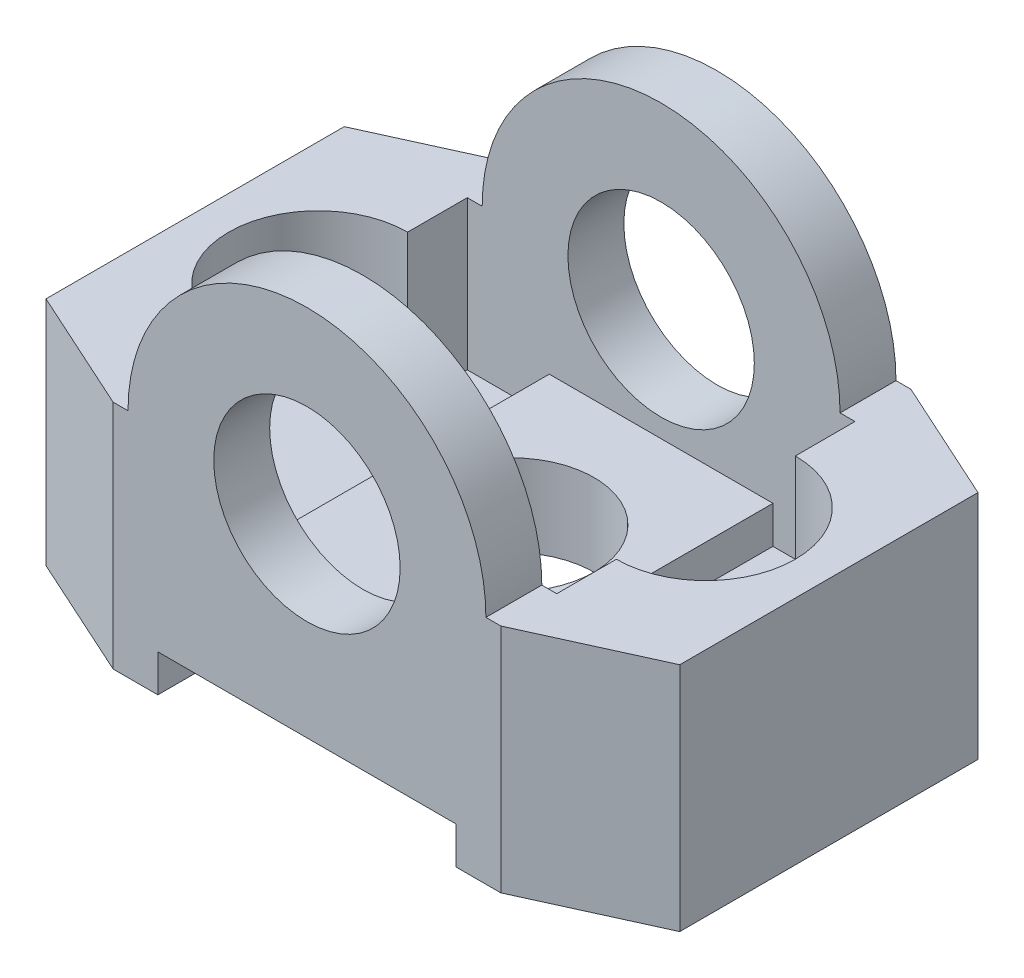
ISO-10303-21;
HEADER;
FILE_DESCRIPTION(('STEP AP214'),'2;1');
FILE_NAME('part.step','',(''),(''),'','','');
FILE_SCHEMA(('AUTOMOTIVE_DESIGN { 1 0 10303 214 1 1 1 1 }'));
ENDSEC;
DATA;
#1=APPLICATION_CONTEXT('core data for automotive mechanical design processes');
#2=APPLICATION_PROTOCOL_DEFINITION('international standard','automotive_design',2000,#1);
#3=PRODUCT_CONTEXT('',#1,'mechanical');
#4=PRODUCT('Part','Part','',(#3));
#5=PRODUCT_RELATED_PRODUCT_CATEGORY('part','',(#4));
#6=PRODUCT_DEFINITION_FORMATION('','',#4);
#7=PRODUCT_DEFINITION_CONTEXT('part definition',#1,'design');
#8=PRODUCT_DEFINITION('design','',#6,#7);
#9=PRODUCT_DEFINITION_SHAPE('','',#8);
#10=(LENGTH_UNIT() NAMED_UNIT(*) SI_UNIT(.MILLI.,.METRE.));
#11=(NAMED_UNIT(*) PLANE_ANGLE_UNIT() SI_UNIT($,.RADIAN.));
#12=(NAMED_UNIT(*) SI_UNIT($,.STERADIAN.) SOLID_ANGLE_UNIT());
#13=UNCERTAINTY_MEASURE_WITH_UNIT(LENGTH_MEASURE(1.E-05),#10,'distance_accuracy_value','');
#14=(GEOMETRIC_REPRESENTATION_CONTEXT(3) GLOBAL_UNCERTAINTY_ASSIGNED_CONTEXT((#13)) GLOBAL_UNIT_ASSIGNED_CONTEXT((#10,
#11,#12)) REPRESENTATION_CONTEXT('',''));
#15=CARTESIAN_POINT('',(0.,0.,0.));
#16=DIRECTION('',(0.,0.,1.));
#17=DIRECTION('',(1.,0.,0.));
#18=AXIS2_PLACEMENT_3D('',#15,#16,#17);
#19=CARTESIAN_POINT('',(0.,0.,0.));
#20=DIRECTION('',(0.,-1.,0.));
#21=DIRECTION('',(0.,0.,-1.));
#22=AXIS2_PLACEMENT_3D('',#19,#20,#21);
#23=PLANE('',#22);
#24=DIRECTION('',(0.,0.,1.));
#25=VECTOR('',#24,1.);
#26=CARTESIAN_POINT('',(-20.,0.,-27.501));
#27=LINE('',#26,#25);
#28=CARTESIAN_POINT('',(-20.,0.,-27.5));
#29=VERTEX_POINT('',#28);
#30=CARTESIAN_POINT('',(-20.,0.,27.5));
#31=VERTEX_POINT('',#30);
#32=EDGE_CURVE('E223',#29,#31,#27,.T.);
#33=ORIENTED_EDGE('',*,*,#32,.T.);
#34=DIRECTION('',(1.,0.,0.));
#35=VECTOR('',#34,1.);
#36=CARTESIAN_POINT('',(26.,0.,27.5));
#37=LINE('',#36,#35);
#38=CARTESIAN_POINT('',(-26.,0.,27.5));
#39=VERTEX_POINT('',#38);
#40=EDGE_CURVE('E267',#39,#31,#37,.T.);
#41=ORIENTED_EDGE('',*,*,#40,.F.);
#42=DIRECTION('',(0.910366477462604,0.,0.413802944301187));
#43=VECTOR('',#42,1.);
#44=CARTESIAN_POINT('',(-42.5,0.,20.));
#45=LINE('',#44,#43);
#46=CARTESIAN_POINT('',(-42.5,0.,20.));
#47=VERTEX_POINT('',#46);
#48=EDGE_CURVE('E264',#47,#39,#45,.T.);
#49=ORIENTED_EDGE('',*,*,#48,.F.);
#50=DIRECTION('',(0.,0.,1.));
#51=VECTOR('',#50,1.);
#52=CARTESIAN_POINT('',(-42.5,0.,-20.));
#53=LINE('',#52,#51);
#54=CARTESIAN_POINT('',(-42.5,0.,-20.));
#55=VERTEX_POINT('',#54);
#56=EDGE_CURVE('E265',#55,#47,#53,.T.);
#57=ORIENTED_EDGE('',*,*,#56,.F.);
#58=DIRECTION('',(-0.910366477462604,0.,0.413802944301186));
#59=VECTOR('',#58,1.);
#60=CARTESIAN_POINT('',(-26.,0.,-27.5));
#61=LINE('',#60,#59);
#62=CARTESIAN_POINT('',(-26.,0.,-27.5));
#63=VERTEX_POINT('',#62);
#64=EDGE_CURVE('E253',#63,#55,#61,.T.);
#65=ORIENTED_EDGE('',*,*,#64,.F.);
#66=DIRECTION('',(-1.,0.,0.));
#67=VECTOR('',#66,1.);
#68=CARTESIAN_POINT('',(-26.,0.,-27.5));
#69=LINE('',#68,#67);
#70=EDGE_CURVE('E244',#29,#63,#69,.T.);
#71=ORIENTED_EDGE('',*,*,#70,.F.);
#72=EDGE_LOOP('',(#33,#41,#49,#57,#65,#71));
#73=FACE_BOUND('',#72,.T.);
#74=ADVANCED_FACE('F39',(#73),#23,.T.);
#75=CARTESIAN_POINT('',(-26.,31.,-20.));
#76=DIRECTION('',(0.,0.,1.));
#77=DIRECTION('',(1.,0.,0.));
#78=AXIS2_PLACEMENT_3D('',#75,#76,#77);
#79=PLANE('',#78);
#80=CARTESIAN_POINT('',(0.,31.,-20.));
#81=DIRECTION('',(0.,0.,1.));
#82=DIRECTION('',(1.,0.,0.));
#83=AXIS2_PLACEMENT_3D('',#80,#81,#82);
#84=CIRCLE('',#83,12.5);
#85=CARTESIAN_POINT('',(12.5,31.,-20.));
#86=VERTEX_POINT('',#85);
#87=EDGE_CURVE('E297',#86,#86,#84,.T.);
#88=ORIENTED_EDGE('',*,*,#87,.F.);
#89=EDGE_LOOP('',(#88));
#90=FACE_BOUND('',#89,.T.);
#91=DIRECTION('',(-1.,0.,0.));
#92=VECTOR('',#91,1.);
#93=CARTESIAN_POINT('',(-15.,16.,-20.));
#94=LINE('',#93,#92);
#95=CARTESIAN_POINT('',(15.,16.,-20.));
#96=VERTEX_POINT('',#95);
#97=CARTESIAN_POINT('',(-15.,16.,-20.));
#98=VERTEX_POINT('',#97);
#99=EDGE_CURVE('E422',#96,#98,#94,.T.);
#100=ORIENTED_EDGE('',*,*,#99,.F.);
#101=DIRECTION('',(0.,-1.,0.));
#102=VECTOR('',#101,1.);
#103=CARTESIAN_POINT('',(15.,16.,-20.));
#104=LINE('',#103,#102);
#105=CARTESIAN_POINT('',(15.,11.,-20.));
#106=VERTEX_POINT('',#105);
#107=EDGE_CURVE('E439',#96,#106,#104,.T.);
#108=ORIENTED_EDGE('',*,*,#107,.T.);
#109=DIRECTION('',(-1.,0.,0.));
#110=VECTOR('',#109,1.);
#111=CARTESIAN_POINT('',(-26.,11.,-20.));
#112=LINE('',#111,#110);
#113=CARTESIAN_POINT('',(26.,11.,-20.));
#114=VERTEX_POINT('',#113);
#115=EDGE_CURVE('E459',#114,#106,#112,.T.);
#116=ORIENTED_EDGE('',*,*,#115,.F.);
#117=DIRECTION('',(0.,-1.,0.));
#118=VECTOR('',#117,1.);
#119=CARTESIAN_POINT('',(26.,31.,-20.));
#120=LINE('',#119,#118);
#121=CARTESIAN_POINT('',(26.,31.,-20.));
#122=VERTEX_POINT('',#121);
#123=EDGE_CURVE('E260',#122,#114,#120,.T.);
#124=ORIENTED_EDGE('',*,*,#123,.F.);
#125=DIRECTION('',(-1.,0.,0.));
#126=VECTOR('',#125,1.);
#127=CARTESIAN_POINT('',(-26.,31.,-20.));
#128=LINE('',#127,#126);
#129=CARTESIAN_POINT('',(24.,31.,-20.));
#130=VERTEX_POINT('',#129);
#131=EDGE_CURVE('E337',#122,#130,#128,.T.);
#132=ORIENTED_EDGE('',*,*,#131,.T.);
#133=CARTESIAN_POINT('',(0.,31.,-20.));
#134=DIRECTION('',(0.,0.,1.));
#135=DIRECTION('',(1.,0.,0.));
#136=AXIS2_PLACEMENT_3D('',#133,#134,#135);
#137=CIRCLE('',#136,24.);
#138=CARTESIAN_POINT('',(-24.,31.,-20.));
#139=VERTEX_POINT('',#138);
#140=EDGE_CURVE('E320',#139,#130,#137,.F.);
#141=ORIENTED_EDGE('',*,*,#140,.F.);
#142=CARTESIAN_POINT('',(-26.,31.,-20.));
#143=VERTEX_POINT('',#142);
#144=EDGE_CURVE('E333',#139,#143,#128,.T.);
#145=ORIENTED_EDGE('',*,*,#144,.T.);
#146=DIRECTION('',(0.,-1.,0.));
#147=VECTOR('',#146,1.);
#148=CARTESIAN_POINT('',(-26.,31.,-20.));
#149=LINE('',#148,#147);
#150=CARTESIAN_POINT('',(-26.,11.,-20.));
#151=VERTEX_POINT('',#150);
#152=EDGE_CURVE('E371',#143,#151,#149,.T.);
#153=ORIENTED_EDGE('',*,*,#152,.T.);
#154=CARTESIAN_POINT('',(-15.,11.,-20.));
#155=VERTEX_POINT('',#154);
#156=EDGE_CURVE('E456',#155,#151,#112,.T.);
#157=ORIENTED_EDGE('',*,*,#156,.F.);
#158=DIRECTION('',(0.,-1.,0.));
#159=VECTOR('',#158,1.);
#160=CARTESIAN_POINT('',(-15.,16.,-20.));
#161=LINE('',#160,#159);
#162=EDGE_CURVE('E64',#98,#155,#161,.T.);
#163=ORIENTED_EDGE('',*,*,#162,.F.);
#164=EDGE_LOOP('',(#100,#108,#116,#124,#132,#141,#145,#153,#157,#163));
#165=FACE_BOUND('',#164,.T.);
#166=ADVANCED_FACE('F474',(#90,#165),#79,.T.);
#167=CARTESIAN_POINT('',(26.,31.,20.));
#168=DIRECTION('',(0.,0.,-1.));
#169=DIRECTION('',(-1.,0.,0.));
#170=AXIS2_PLACEMENT_3D('',#167,#168,#169);
#171=PLANE('',#170);
#172=CARTESIAN_POINT('',(0.,31.,20.));
#173=DIRECTION('',(0.,0.,-1.));
#174=DIRECTION('',(-1.,0.,0.));
#175=AXIS2_PLACEMENT_3D('',#172,#173,#174);
#176=CIRCLE('',#175,12.5);
#177=CARTESIAN_POINT('',(-12.5,31.,20.));
#178=VERTEX_POINT('',#177);
#179=EDGE_CURVE('E294',#178,#178,#176,.T.);
#180=ORIENTED_EDGE('',*,*,#179,.F.);
#181=EDGE_LOOP('',(#180));
#182=FACE_BOUND('',#181,.T.);
#183=DIRECTION('',(1.,0.,0.));
#184=VECTOR('',#183,1.);
#185=CARTESIAN_POINT('',(26.,11.,20.));
#186=LINE('',#185,#184);
#187=CARTESIAN_POINT('',(15.,11.,20.));
#188=VERTEX_POINT('',#187);
#189=CARTESIAN_POINT('',(26.,11.,20.));
#190=VERTEX_POINT('',#189);
#191=EDGE_CURVE('E447',#188,#190,#186,.T.);
#192=ORIENTED_EDGE('',*,*,#191,.F.);
#193=DIRECTION('',(0.,-1.,0.));
#194=VECTOR('',#193,1.);
#195=CARTESIAN_POINT('',(15.,16.,20.));
#196=LINE('',#195,#194);
#197=CARTESIAN_POINT('',(15.,16.,20.));
#198=VERTEX_POINT('',#197);
#199=EDGE_CURVE('E435',#198,#188,#196,.T.);
#200=ORIENTED_EDGE('',*,*,#199,.F.);
#201=DIRECTION('',(1.,0.,0.));
#202=VECTOR('',#201,1.);
#203=CARTESIAN_POINT('',(-15.,16.,20.));
#204=LINE('',#203,#202);
#205=CARTESIAN_POINT('',(-15.,16.,20.));
#206=VERTEX_POINT('',#205);
#207=EDGE_CURVE('E429',#206,#198,#204,.T.);
#208=ORIENTED_EDGE('',*,*,#207,.F.);
#209=DIRECTION('',(0.,-1.,0.));
#210=VECTOR('',#209,1.);
#211=CARTESIAN_POINT('',(-15.,16.,20.));
#212=LINE('',#211,#210);
#213=CARTESIAN_POINT('',(-15.,11.,20.));
#214=VERTEX_POINT('',#213);
#215=EDGE_CURVE('E436',#206,#214,#212,.T.);
#216=ORIENTED_EDGE('',*,*,#215,.T.);
#217=CARTESIAN_POINT('',(-26.,11.,20.));
#218=VERTEX_POINT('',#217);
#219=EDGE_CURVE('E449',#218,#214,#186,.T.);
#220=ORIENTED_EDGE('',*,*,#219,.F.);
#221=DIRECTION('',(0.,-1.,0.));
#222=VECTOR('',#221,1.);
#223=CARTESIAN_POINT('',(-26.,31.,20.));
#224=LINE('',#223,#222);
#225=CARTESIAN_POINT('',(-26.,31.,20.));
#226=VERTEX_POINT('',#225);
#227=EDGE_CURVE('E362',#226,#218,#224,.T.);
#228=ORIENTED_EDGE('',*,*,#227,.F.);
#229=DIRECTION('',(1.,0.,0.));
#230=VECTOR('',#229,1.);
#231=CARTESIAN_POINT('',(26.,31.,20.));
#232=LINE('',#231,#230);
#233=CARTESIAN_POINT('',(-24.,31.,20.));
#234=VERTEX_POINT('',#233);
#235=EDGE_CURVE('E347',#226,#234,#232,.T.);
#236=ORIENTED_EDGE('',*,*,#235,.T.);
#237=CARTESIAN_POINT('',(0.,31.,20.));
#238=DIRECTION('',(0.,0.,-1.));
#239=DIRECTION('',(-1.,0.,0.));
#240=AXIS2_PLACEMENT_3D('',#237,#238,#239);
#241=CIRCLE('',#240,24.);
#242=CARTESIAN_POINT('',(24.,31.,20.));
#243=VERTEX_POINT('',#242);
#244=EDGE_CURVE('E330',#243,#234,#241,.F.);
#245=ORIENTED_EDGE('',*,*,#244,.F.);
#246=CARTESIAN_POINT('',(26.,31.,20.));
#247=VERTEX_POINT('',#246);
#248=EDGE_CURVE('E341',#243,#247,#232,.T.);
#249=ORIENTED_EDGE('',*,*,#248,.T.);
#250=DIRECTION('',(0.,-1.,0.));
#251=VECTOR('',#250,1.);
#252=CARTESIAN_POINT('',(26.,31.,20.));
#253=LINE('',#252,#251);
#254=EDGE_CURVE('E359',#247,#190,#253,.T.);
#255=ORIENTED_EDGE('',*,*,#254,.T.);
#256=EDGE_LOOP('',(#192,#200,#208,#216,#220,#228,#236,#245,#249,#255));
#257=FACE_BOUND('',#256,.T.);
#258=ADVANCED_FACE('F495',(#182,#257),#171,.T.);
#259=CARTESIAN_POINT('',(0.,11.,0.));
#260=DIRECTION('',(0.,1.,0.));
#261=DIRECTION('',(0.,0.,1.));
#262=AXIS2_PLACEMENT_3D('',#259,#260,#261);
#263=PLANE('',#262);
#264=ORIENTED_EDGE('',*,*,#115,.T.);
#265=DIRECTION('',(0.,0.,-1.));
#266=VECTOR('',#265,1.);
#267=CARTESIAN_POINT('',(15.,11.,20.));
#268=LINE('',#267,#266);
#269=EDGE_CURVE('E423',#188,#106,#268,.T.);
#270=ORIENTED_EDGE('',*,*,#269,.F.);
#271=ORIENTED_EDGE('',*,*,#191,.T.);
#272=DIRECTION('',(0.,0.,-1.));
#273=VECTOR('',#272,1.);
#274=CARTESIAN_POINT('',(26.,11.,12.));
#275=LINE('',#274,#273);
#276=CARTESIAN_POINT('',(26.,11.,12.));
#277=VERTEX_POINT('',#276);
#278=EDGE_CURVE('E444',#190,#277,#275,.T.);
#279=ORIENTED_EDGE('',*,*,#278,.T.);
#280=CARTESIAN_POINT('',(26.,11.,0.));
#281=DIRECTION('',(0.,1.,0.));
#282=DIRECTION('',(0.,0.,1.));
#283=AXIS2_PLACEMENT_3D('',#280,#281,#282);
#284=CIRCLE('',#283,12.);
#285=CARTESIAN_POINT('',(26.,11.,-12.));
#286=VERTEX_POINT('',#285);
#287=EDGE_CURVE('E11',#277,#286,#284,.T.);
#288=ORIENTED_EDGE('',*,*,#287,.T.);
#289=DIRECTION('',(0.,0.,-1.));
#290=VECTOR('',#289,1.);
#291=CARTESIAN_POINT('',(26.,11.,-20.));
#292=LINE('',#291,#290);
#293=EDGE_CURVE('E310',#286,#114,#292,.T.);
#294=ORIENTED_EDGE('',*,*,#293,.T.);
#295=EDGE_LOOP('',(#264,#270,#271,#279,#288,#294));
#296=FACE_BOUND('',#295,.T.);
#297=ADVANCED_FACE('F516',(#296),#263,.T.);
#298=ORIENTED_EDGE('',*,*,#219,.T.);
#299=DIRECTION('',(0.,0.,1.));
#300=VECTOR('',#299,1.);
#301=CARTESIAN_POINT('',(-15.,11.,20.));
#302=LINE('',#301,#300);
#303=EDGE_CURVE('E426',#155,#214,#302,.T.);
#304=ORIENTED_EDGE('',*,*,#303,.F.);
#305=ORIENTED_EDGE('',*,*,#156,.T.);
#306=DIRECTION('',(0.,0.,1.));
#307=VECTOR('',#306,1.);
#308=CARTESIAN_POINT('',(-26.,11.,-12.));
#309=LINE('',#308,#307);
#310=CARTESIAN_POINT('',(-26.,11.,-12.));
#311=VERTEX_POINT('',#310);
#312=EDGE_CURVE('E457',#151,#311,#309,.T.);
#313=ORIENTED_EDGE('',*,*,#312,.T.);
#314=CARTESIAN_POINT('',(-26.,11.,0.));
#315=DIRECTION('',(0.,1.,0.));
#316=DIRECTION('',(0.,0.,1.));
#317=AXIS2_PLACEMENT_3D('',#314,#315,#316);
#318=CIRCLE('',#317,12.);
#319=CARTESIAN_POINT('',(-26.,11.,12.));
#320=VERTEX_POINT('',#319);
#321=EDGE_CURVE('E453',#311,#320,#318,.T.);
#322=ORIENTED_EDGE('',*,*,#321,.T.);
#323=DIRECTION('',(0.,0.,1.));
#324=VECTOR('',#323,1.);
#325=CARTESIAN_POINT('',(-26.,11.,20.));
#326=LINE('',#325,#324);
#327=EDGE_CURVE('E448',#320,#218,#326,.T.);
#328=ORIENTED_EDGE('',*,*,#327,.T.);
#329=EDGE_LOOP('',(#298,#304,#305,#313,#322,#328));
#330=FACE_BOUND('',#329,.T.);
#331=ADVANCED_FACE('F470',(#330),#263,.T.);
#332=CARTESIAN_POINT('',(0.,31.,0.));
#333=DIRECTION('',(0.,-1.,0.));
#334=DIRECTION('',(0.,0.,-1.));
#335=AXIS2_PLACEMENT_3D('',#332,#333,#334);
#336=PLANE('',#335);
#337=ORIENTED_EDGE('',*,*,#144,.F.);
#338=DIRECTION('',(0.,0.,-1.));
#339=VECTOR('',#338,1.);
#340=CARTESIAN_POINT('',(-24.,31.,33.665631459995));
#341=LINE('',#340,#339);
#342=CARTESIAN_POINT('',(-24.,31.,-27.5));
#343=VERTEX_POINT('',#342);
#344=EDGE_CURVE('E316',#139,#343,#341,.T.);
#345=ORIENTED_EDGE('',*,*,#344,.T.);
#346=DIRECTION('',(-1.,0.,0.));
#347=VECTOR('',#346,1.);
#348=CARTESIAN_POINT('',(-26.,31.,-27.5));
#349=LINE('',#348,#347);
#350=CARTESIAN_POINT('',(-26.,31.,-27.5));
#351=VERTEX_POINT('',#350);
#352=EDGE_CURVE('E378',#343,#351,#349,.T.);
#353=ORIENTED_EDGE('',*,*,#352,.T.);
#354=DIRECTION('',(-0.910366477462604,0.,0.413802944301186));
#355=VECTOR('',#354,1.);
#356=CARTESIAN_POINT('',(-26.,31.,-27.5));
#357=LINE('',#356,#355);
#358=CARTESIAN_POINT('',(-42.5,31.,-20.));
#359=VERTEX_POINT('',#358);
#360=EDGE_CURVE('E385',#351,#359,#357,.T.);
#361=ORIENTED_EDGE('',*,*,#360,.T.);
#362=DIRECTION('',(0.,0.,1.));
#363=VECTOR('',#362,1.);
#364=CARTESIAN_POINT('',(-42.5,31.,-20.));
#365=LINE('',#364,#363);
#366=CARTESIAN_POINT('',(-42.5,31.,20.));
#367=VERTEX_POINT('',#366);
#368=EDGE_CURVE('E383',#359,#367,#365,.T.);
#369=ORIENTED_EDGE('',*,*,#368,.T.);
#370=DIRECTION('',(0.910366477462604,0.,0.413802944301187));
#371=VECTOR('',#370,1.);
#372=CARTESIAN_POINT('',(-42.5,31.,20.));
#373=LINE('',#372,#371);
#374=CARTESIAN_POINT('',(-26.,31.,27.5));
#375=VERTEX_POINT('',#374);
#376=EDGE_CURVE('E387',#367,#375,#373,.T.);
#377=ORIENTED_EDGE('',*,*,#376,.T.);
#378=DIRECTION('',(1.,0.,0.));
#379=VECTOR('',#378,1.);
#380=CARTESIAN_POINT('',(26.,31.,27.5));
#381=LINE('',#380,#379);
#382=CARTESIAN_POINT('',(-24.,31.,27.5));
#383=VERTEX_POINT('',#382);
#384=EDGE_CURVE('E386',#375,#383,#381,.T.);
#385=ORIENTED_EDGE('',*,*,#384,.T.);
#386=DIRECTION('',(0.,0.,1.));
#387=VECTOR('',#386,1.);
#388=CARTESIAN_POINT('',(-24.,31.,-33.6656314599949));
#389=LINE('',#388,#387);
#390=EDGE_CURVE('E328',#234,#383,#389,.T.);
#391=ORIENTED_EDGE('',*,*,#390,.F.);
#392=ORIENTED_EDGE('',*,*,#235,.F.);
#393=DIRECTION('',(0.,0.,1.));
#394=VECTOR('',#393,1.);
#395=CARTESIAN_POINT('',(-26.,31.,20.));
#396=LINE('',#395,#394);
#397=CARTESIAN_POINT('',(-26.,31.,12.));
#398=VERTEX_POINT('',#397);
#399=EDGE_CURVE('E343',#398,#226,#396,.T.);
#400=ORIENTED_EDGE('',*,*,#399,.F.);
#401=CARTESIAN_POINT('',(-26.,31.,0.));
#402=DIRECTION('',(0.,1.,0.));
#403=DIRECTION('',(0.,0.,1.));
#404=AXIS2_PLACEMENT_3D('',#401,#402,#403);
#405=CIRCLE('',#404,12.);
#406=CARTESIAN_POINT('',(-26.,31.,-12.));
#407=VERTEX_POINT('',#406);
#408=EDGE_CURVE('E342',#407,#398,#405,.T.);
#409=ORIENTED_EDGE('',*,*,#408,.F.);
#410=DIRECTION('',(0.,0.,1.));
#411=VECTOR('',#410,1.);
#412=CARTESIAN_POINT('',(-26.,31.,-12.));
#413=LINE('',#412,#411);
#414=EDGE_CURVE('E336',#143,#407,#413,.T.);
#415=ORIENTED_EDGE('',*,*,#414,.F.);
#416=EDGE_LOOP('',(#337,#345,#353,#361,#369,#377,#385,#391,#392,#400,#409,#415));
#417=FACE_BOUND('',#416,.T.);
#418=ADVANCED_FACE('F479',(#417),#336,.F.);
#419=CARTESIAN_POINT('',(26.,31.,-27.5));
#420=VERTEX_POINT('',#419);
#421=CARTESIAN_POINT('',(24.,31.,-27.5));
#422=VERTEX_POINT('',#421);
#423=EDGE_CURVE('E377',#420,#422,#349,.T.);
#424=ORIENTED_EDGE('',*,*,#423,.T.);
#425=DIRECTION('',(0.,0.,-1.));
#426=VECTOR('',#425,1.);
#427=CARTESIAN_POINT('',(24.,31.,33.665631459995));
#428=LINE('',#427,#426);
#429=EDGE_CURVE('E317',#130,#422,#428,.T.);
#430=ORIENTED_EDGE('',*,*,#429,.F.);
#431=ORIENTED_EDGE('',*,*,#131,.F.);
#432=DIRECTION('',(0.,0.,-1.));
#433=VECTOR('',#432,1.);
#434=CARTESIAN_POINT('',(26.,31.,-20.));
#435=LINE('',#434,#433);
#436=CARTESIAN_POINT('',(26.,31.,-12.));
#437=VERTEX_POINT('',#436);
#438=EDGE_CURVE('E334',#437,#122,#435,.T.);
#439=ORIENTED_EDGE('',*,*,#438,.F.);
#440=CARTESIAN_POINT('',(26.,31.,0.));
#441=DIRECTION('',(0.,1.,0.));
#442=DIRECTION('',(0.,0.,-1.));
#443=AXIS2_PLACEMENT_3D('',#440,#441,#442);
#444=CIRCLE('',#443,12.);
#445=CARTESIAN_POINT('',(26.,31.,12.));
#446=VERTEX_POINT('',#445);
#447=EDGE_CURVE('E354',#446,#437,#444,.T.);
#448=ORIENTED_EDGE('',*,*,#447,.F.);
#449=DIRECTION('',(0.,0.,-1.));
#450=VECTOR('',#449,1.);
#451=CARTESIAN_POINT('',(26.,31.,12.));
#452=LINE('',#451,#450);
#453=EDGE_CURVE('E349',#247,#446,#452,.T.);
#454=ORIENTED_EDGE('',*,*,#453,.F.);
#455=ORIENTED_EDGE('',*,*,#248,.F.);
#456=DIRECTION('',(0.,0.,1.));
#457=VECTOR('',#456,1.);
#458=CARTESIAN_POINT('',(24.,31.,-33.6656314599949));
#459=LINE('',#458,#457);
#460=CARTESIAN_POINT('',(24.,31.,27.5));
#461=VERTEX_POINT('',#460);
#462=EDGE_CURVE('E326',#243,#461,#459,.T.);
#463=ORIENTED_EDGE('',*,*,#462,.T.);
#464=CARTESIAN_POINT('',(26.,31.,27.5));
#465=VERTEX_POINT('',#464);
#466=EDGE_CURVE('E389',#461,#465,#381,.T.);
#467=ORIENTED_EDGE('',*,*,#466,.T.);
#468=DIRECTION('',(0.910366477462605,0.,-0.413802944301184));
#469=VECTOR('',#468,1.);
#470=CARTESIAN_POINT('',(42.5,31.,20.));
#471=LINE('',#470,#469);
#472=CARTESIAN_POINT('',(42.5,31.,20.));
#473=VERTEX_POINT('',#472);
#474=EDGE_CURVE('E394',#465,#473,#471,.T.);
#475=ORIENTED_EDGE('',*,*,#474,.T.);
#476=DIRECTION('',(0.,0.,-1.));
#477=VECTOR('',#476,1.);
#478=CARTESIAN_POINT('',(42.5,31.,-20.));
#479=LINE('',#478,#477);
#480=CARTESIAN_POINT('',(42.5,31.,-20.));
#481=VERTEX_POINT('',#480);
#482=EDGE_CURVE('E282',#473,#481,#479,.T.);
#483=ORIENTED_EDGE('',*,*,#482,.T.);
#484=DIRECTION('',(-0.910366477462604,0.,-0.413802944301186));
#485=VECTOR('',#484,1.);
#486=CARTESIAN_POINT('',(26.,31.,-27.5));
#487=LINE('',#486,#485);
#488=EDGE_CURVE('E280',#481,#420,#487,.T.);
#489=ORIENTED_EDGE('',*,*,#488,.T.);
#490=EDGE_LOOP('',(#424,#430,#431,#439,#448,#454,#455,#463,#467,#475,#483,#489));
#491=FACE_BOUND('',#490,.T.);
#492=ADVANCED_FACE('F397',(#491),#336,.F.);
#493=DIRECTION('',(0.,0.,1.));
#494=VECTOR('',#493,1.);
#495=CARTESIAN_POINT('',(20.,0.,-27.501));
#496=LINE('',#495,#494);
#497=CARTESIAN_POINT('',(20.,0.,-27.5));
#498=VERTEX_POINT('',#497);
#499=CARTESIAN_POINT('',(20.,0.,27.5));
#500=VERTEX_POINT('',#499);
#501=EDGE_CURVE('E237',#498,#500,#496,.T.);
#502=ORIENTED_EDGE('',*,*,#501,.F.);
#503=CARTESIAN_POINT('',(26.,0.,-27.5));
#504=VERTEX_POINT('',#503);
#505=EDGE_CURVE('E252',#504,#498,#69,.T.);
#506=ORIENTED_EDGE('',*,*,#505,.F.);
#507=DIRECTION('',(-0.910366477462604,0.,-0.413802944301186));
#508=VECTOR('',#507,1.);
#509=CARTESIAN_POINT('',(26.,0.,-27.5));
#510=LINE('',#509,#508);
#511=CARTESIAN_POINT('',(42.5,0.,-20.));
#512=VERTEX_POINT('',#511);
#513=EDGE_CURVE('E251',#512,#504,#510,.T.);
#514=ORIENTED_EDGE('',*,*,#513,.F.);
#515=DIRECTION('',(0.,0.,-1.));
#516=VECTOR('',#515,1.);
#517=CARTESIAN_POINT('',(42.5,0.,-20.));
#518=LINE('',#517,#516);
#519=CARTESIAN_POINT('',(42.5,0.,20.));
#520=VERTEX_POINT('',#519);
#521=EDGE_CURVE('E273',#520,#512,#518,.T.);
#522=ORIENTED_EDGE('',*,*,#521,.F.);
#523=DIRECTION('',(0.910366477462605,0.,-0.413802944301184));
#524=VECTOR('',#523,1.);
#525=CARTESIAN_POINT('',(42.5,0.,20.));
#526=LINE('',#525,#524);
#527=CARTESIAN_POINT('',(26.,0.,27.5));
#528=VERTEX_POINT('',#527);
#529=EDGE_CURVE('E271',#528,#520,#526,.T.);
#530=ORIENTED_EDGE('',*,*,#529,.F.);
#531=EDGE_CURVE('E268',#500,#528,#37,.T.);
#532=ORIENTED_EDGE('',*,*,#531,.F.);
#533=EDGE_LOOP('',(#502,#506,#514,#522,#530,#532));
#534=FACE_BOUND('',#533,.T.);
#535=ADVANCED_FACE('F406',(#534),#23,.T.);
#536=CARTESIAN_POINT('',(26.,31.,-27.5));
#537=DIRECTION('',(-0.413802944301186,0.,0.910366477462604));
#538=DIRECTION('',(0.910366477462604,0.,0.413802944301186));
#539=AXIS2_PLACEMENT_3D('',#536,#537,#538);
#540=PLANE('',#539);
#541=DIRECTION('',(0.,-1.,0.));
#542=VECTOR('',#541,1.);
#543=CARTESIAN_POINT('',(42.5,31.,-20.));
#544=LINE('',#543,#542);
#545=EDGE_CURVE('E279',#481,#512,#544,.T.);
#546=ORIENTED_EDGE('',*,*,#545,.T.);
#547=ORIENTED_EDGE('',*,*,#513,.T.);
#548=DIRECTION('',(0.,-1.,0.));
#549=VECTOR('',#548,1.);
#550=CARTESIAN_POINT('',(26.,31.,-27.5));
#551=LINE('',#550,#549);
#552=EDGE_CURVE('E50',#420,#504,#551,.T.);
#553=ORIENTED_EDGE('',*,*,#552,.F.);
#554=ORIENTED_EDGE('',*,*,#488,.F.);
#555=EDGE_LOOP('',(#546,#547,#553,#554));
#556=FACE_BOUND('',#555,.T.);
#557=ADVANCED_FACE('F41',(#556),#540,.F.);
#558=CARTESIAN_POINT('',(-26.,31.,-27.5));
#559=DIRECTION('',(0.,0.,1.));
#560=DIRECTION('',(1.,0.,0.));
#561=AXIS2_PLACEMENT_3D('',#558,#559,#560);
#562=PLANE('',#561);
#563=CARTESIAN_POINT('',(0.,31.,-27.5));
#564=DIRECTION('',(0.,0.,1.));
#565=DIRECTION('',(1.,0.,0.));
#566=AXIS2_PLACEMENT_3D('',#563,#564,#565);
#567=CIRCLE('',#566,12.5);
#568=CARTESIAN_POINT('',(12.5,31.,-27.5));
#569=VERTEX_POINT('',#568);
#570=EDGE_CURVE('E299',#569,#569,#567,.T.);
#571=ORIENTED_EDGE('',*,*,#570,.T.);
#572=EDGE_LOOP('',(#571));
#573=FACE_BOUND('',#572,.T.);
#574=DIRECTION('',(1.,0.,0.));
#575=VECTOR('',#574,1.);
#576=CARTESIAN_POINT('',(-20.,5.,-27.5));
#577=LINE('',#576,#575);
#578=CARTESIAN_POINT('',(-20.,5.,-27.5));
#579=VERTEX_POINT('',#578);
#580=CARTESIAN_POINT('',(20.,5.,-27.5));
#581=VERTEX_POINT('',#580);
#582=EDGE_CURVE('E247',#579,#581,#577,.T.);
#583=ORIENTED_EDGE('',*,*,#582,.F.);
#584=DIRECTION('',(0.,1.,0.));
#585=VECTOR('',#584,1.);
#586=CARTESIAN_POINT('',(-20.,0.,-27.5));
#587=LINE('',#586,#585);
#588=EDGE_CURVE('E230',#29,#579,#587,.T.);
#589=ORIENTED_EDGE('',*,*,#588,.F.);
#590=ORIENTED_EDGE('',*,*,#70,.T.);
#591=DIRECTION('',(0.,-1.,0.));
#592=VECTOR('',#591,1.);
#593=CARTESIAN_POINT('',(-26.,31.,-27.5));
#594=LINE('',#593,#592);
#595=EDGE_CURVE('E295',#351,#63,#594,.T.);
#596=ORIENTED_EDGE('',*,*,#595,.F.);
#597=ORIENTED_EDGE('',*,*,#352,.F.);
#598=CARTESIAN_POINT('',(0.,31.,-27.5));
#599=DIRECTION('',(0.,0.,-1.));
#600=DIRECTION('',(1.,0.,0.));
#601=AXIS2_PLACEMENT_3D('',#598,#599,#600);
#602=CIRCLE('',#601,24.);
#603=EDGE_CURVE('E302',#343,#422,#602,.T.);
#604=ORIENTED_EDGE('',*,*,#603,.T.);
#605=ORIENTED_EDGE('',*,*,#423,.F.);
#606=ORIENTED_EDGE('',*,*,#552,.T.);
#607=ORIENTED_EDGE('',*,*,#505,.T.);
#608=DIRECTION('',(0.,-1.,0.));
#609=VECTOR('',#608,1.);
#610=CARTESIAN_POINT('',(20.,0.,-27.5));
#611=LINE('',#610,#609);
#612=EDGE_CURVE('E664',#581,#498,#611,.T.);
#613=ORIENTED_EDGE('',*,*,#612,.F.);
#614=EDGE_LOOP('',(#583,#589,#590,#596,#597,#604,#605,#606,#607,#613));
#615=FACE_BOUND('',#614,.T.);
#616=ADVANCED_FACE('F238',(#573,#615),#562,.F.);
#617=CARTESIAN_POINT('',(-26.,31.,-27.5));
#618=DIRECTION('',(0.413802944301186,0.,0.910366477462604));
#619=DIRECTION('',(0.910366477462604,0.,-0.413802944301186));
#620=AXIS2_PLACEMENT_3D('',#617,#618,#619);
#621=PLANE('',#620);
#622=ORIENTED_EDGE('',*,*,#595,.T.);
#623=ORIENTED_EDGE('',*,*,#64,.T.);
#624=DIRECTION('',(0.,-1.,0.));
#625=VECTOR('',#624,1.);
#626=CARTESIAN_POINT('',(-42.5,31.,-20.));
#627=LINE('',#626,#625);
#628=EDGE_CURVE('E286',#359,#55,#627,.T.);
#629=ORIENTED_EDGE('',*,*,#628,.F.);
#630=ORIENTED_EDGE('',*,*,#360,.F.);
#631=EDGE_LOOP('',(#622,#623,#629,#630));
#632=FACE_BOUND('',#631,.T.);
#633=ADVANCED_FACE('F684',(#632),#621,.F.);
#634=CARTESIAN_POINT('',(-42.5,31.,-20.));
#635=DIRECTION('',(1.,0.,0.));
#636=DIRECTION('',(0.,0.,-1.));
#637=AXIS2_PLACEMENT_3D('',#634,#635,#636);
#638=PLANE('',#637);
#639=ORIENTED_EDGE('',*,*,#628,.T.);
#640=ORIENTED_EDGE('',*,*,#56,.T.);
#641=DIRECTION('',(0.,-1.,0.));
#642=VECTOR('',#641,1.);
#643=CARTESIAN_POINT('',(-42.5,31.,20.));
#644=LINE('',#643,#642);
#645=EDGE_CURVE('E288',#367,#47,#644,.T.);
#646=ORIENTED_EDGE('',*,*,#645,.F.);
#647=ORIENTED_EDGE('',*,*,#368,.F.);
#648=EDGE_LOOP('',(#639,#640,#646,#647));
#649=FACE_BOUND('',#648,.T.);
#650=ADVANCED_FACE('F676',(#649),#638,.F.);
#651=CARTESIAN_POINT('',(-42.5,31.,20.));
#652=DIRECTION('',(0.413802944301187,0.,-0.910366477462604));
#653=DIRECTION('',(-0.910366477462604,0.,-0.413802944301187));
#654=AXIS2_PLACEMENT_3D('',#651,#652,#653);
#655=PLANE('',#654);
#656=ORIENTED_EDGE('',*,*,#645,.T.);
#657=ORIENTED_EDGE('',*,*,#48,.T.);
#658=DIRECTION('',(0.,-1.,0.));
#659=VECTOR('',#658,1.);
#660=CARTESIAN_POINT('',(-26.,31.,27.5));
#661=LINE('',#660,#659);
#662=EDGE_CURVE('E287',#375,#39,#661,.T.);
#663=ORIENTED_EDGE('',*,*,#662,.F.);
#664=ORIENTED_EDGE('',*,*,#376,.F.);
#665=EDGE_LOOP('',(#656,#657,#663,#664));
#666=FACE_BOUND('',#665,.T.);
#667=ADVANCED_FACE('F673',(#666),#655,.F.);
#668=CARTESIAN_POINT('',(26.,31.,27.5));
#669=DIRECTION('',(0.,0.,-1.));
#670=DIRECTION('',(-1.,0.,0.));
#671=AXIS2_PLACEMENT_3D('',#668,#669,#670);
#672=PLANE('',#671);
#673=ORIENTED_EDGE('',*,*,#40,.T.);
#674=DIRECTION('',(0.,-1.,0.));
#675=VECTOR('',#674,1.);
#676=CARTESIAN_POINT('',(-20.,0.,27.5));
#677=LINE('',#676,#675);
#678=CARTESIAN_POINT('',(-20.,5.,27.5));
#679=VERTEX_POINT('',#678);
#680=EDGE_CURVE('E232',#679,#31,#677,.T.);
#681=ORIENTED_EDGE('',*,*,#680,.F.);
#682=DIRECTION('',(-1.,0.,0.));
#683=VECTOR('',#682,1.);
#684=CARTESIAN_POINT('',(-20.,5.,27.5));
#685=LINE('',#684,#683);
#686=CARTESIAN_POINT('',(20.,5.,27.5));
#687=VERTEX_POINT('',#686);
#688=EDGE_CURVE('E240',#687,#679,#685,.T.);
#689=ORIENTED_EDGE('',*,*,#688,.F.);
#690=DIRECTION('',(0.,1.,0.));
#691=VECTOR('',#690,1.);
#692=CARTESIAN_POINT('',(20.,0.,27.5));
#693=LINE('',#692,#691);
#694=EDGE_CURVE('E53',#500,#687,#693,.T.);
#695=ORIENTED_EDGE('',*,*,#694,.F.);
#696=ORIENTED_EDGE('',*,*,#531,.T.);
#697=DIRECTION('',(0.,-1.,0.));
#698=VECTOR('',#697,1.);
#699=CARTESIAN_POINT('',(26.,31.,27.5));
#700=LINE('',#699,#698);
#701=EDGE_CURVE('E285',#465,#528,#700,.T.);
#702=ORIENTED_EDGE('',*,*,#701,.F.);
#703=ORIENTED_EDGE('',*,*,#466,.F.);
#704=CARTESIAN_POINT('',(0.,31.,27.5));
#705=DIRECTION('',(0.,0.,1.));
#706=DIRECTION('',(1.,0.,0.));
#707=AXIS2_PLACEMENT_3D('',#704,#705,#706);
#708=CIRCLE('',#707,24.);
#709=EDGE_CURVE('E323',#461,#383,#708,.T.);
#710=ORIENTED_EDGE('',*,*,#709,.T.);
#711=ORIENTED_EDGE('',*,*,#384,.F.);
#712=ORIENTED_EDGE('',*,*,#662,.T.);
#713=EDGE_LOOP('',(#673,#681,#689,#695,#696,#702,#703,#710,#711,#712));
#714=FACE_BOUND('',#713,.T.);
#715=CARTESIAN_POINT('',(0.,31.,27.5));
#716=DIRECTION('',(0.,0.,1.));
#717=DIRECTION('',(1.,0.,0.));
#718=AXIS2_PLACEMENT_3D('',#715,#716,#717);
#719=CIRCLE('',#718,12.5);
#720=CARTESIAN_POINT('',(12.5,31.,27.5));
#721=VERTEX_POINT('',#720);
#722=EDGE_CURVE('E304',#721,#721,#719,.T.);
#723=ORIENTED_EDGE('',*,*,#722,.F.);
#724=EDGE_LOOP('',(#723));
#725=FACE_BOUND('',#724,.T.);
#726=ADVANCED_FACE('F498',(#714,#725),#672,.F.);
#727=CARTESIAN_POINT('',(42.5,31.,20.));
#728=DIRECTION('',(-0.413802944301184,0.,-0.910366477462605));
#729=DIRECTION('',(-0.910366477462605,0.,0.413802944301184));
#730=AXIS2_PLACEMENT_3D('',#727,#728,#729);
#731=PLANE('',#730);
#732=ORIENTED_EDGE('',*,*,#701,.T.);
#733=ORIENTED_EDGE('',*,*,#529,.T.);
#734=DIRECTION('',(0.,-1.,0.));
#735=VECTOR('',#734,1.);
#736=CARTESIAN_POINT('',(42.5,31.,20.));
#737=LINE('',#736,#735);
#738=EDGE_CURVE('E278',#473,#520,#737,.T.);
#739=ORIENTED_EDGE('',*,*,#738,.F.);
#740=ORIENTED_EDGE('',*,*,#474,.F.);
#741=EDGE_LOOP('',(#732,#733,#739,#740));
#742=FACE_BOUND('',#741,.T.);
#743=ADVANCED_FACE('F695',(#742),#731,.F.);
#744=CARTESIAN_POINT('',(42.5,31.,-20.));
#745=DIRECTION('',(-1.,0.,0.));
#746=DIRECTION('',(0.,0.,1.));
#747=AXIS2_PLACEMENT_3D('',#744,#745,#746);
#748=PLANE('',#747);
#749=ORIENTED_EDGE('',*,*,#738,.T.);
#750=ORIENTED_EDGE('',*,*,#521,.T.);
#751=ORIENTED_EDGE('',*,*,#545,.F.);
#752=ORIENTED_EDGE('',*,*,#482,.F.);
#753=EDGE_LOOP('',(#749,#750,#751,#752));
#754=FACE_BOUND('',#753,.T.);
#755=ADVANCED_FACE('F405',(#754),#748,.F.);
#756=CARTESIAN_POINT('',(26.,31.,-20.));
#757=DIRECTION('',(-1.,0.,0.));
#758=DIRECTION('',(0.,0.,1.));
#759=AXIS2_PLACEMENT_3D('',#756,#757,#758);
#760=PLANE('',#759);
#761=ORIENTED_EDGE('',*,*,#293,.F.);
#762=DIRECTION('',(0.,-1.,0.));
#763=VECTOR('',#762,1.);
#764=CARTESIAN_POINT('',(26.,31.,-12.));
#765=LINE('',#764,#763);
#766=EDGE_CURVE('E351',#437,#286,#765,.T.);
#767=ORIENTED_EDGE('',*,*,#766,.F.);
#768=ORIENTED_EDGE('',*,*,#438,.T.);
#769=ORIENTED_EDGE('',*,*,#123,.T.);
#770=EDGE_LOOP('',(#761,#767,#768,#769));
#771=FACE_BOUND('',#770,.T.);
#772=ADVANCED_FACE('F519',(#771),#760,.T.);
#773=CARTESIAN_POINT('',(-26.,31.,-12.));
#774=DIRECTION('',(1.,0.,0.));
#775=DIRECTION('',(0.,0.,-1.));
#776=AXIS2_PLACEMENT_3D('',#773,#774,#775);
#777=PLANE('',#776);
#778=ORIENTED_EDGE('',*,*,#312,.F.);
#779=ORIENTED_EDGE('',*,*,#152,.F.);
#780=ORIENTED_EDGE('',*,*,#414,.T.);
#781=DIRECTION('',(0.,-1.,0.));
#782=VECTOR('',#781,1.);
#783=CARTESIAN_POINT('',(-26.,31.,-12.));
#784=LINE('',#783,#782);
#785=EDGE_CURVE('E366',#407,#311,#784,.T.);
#786=ORIENTED_EDGE('',*,*,#785,.T.);
#787=EDGE_LOOP('',(#778,#779,#780,#786));
#788=FACE_BOUND('',#787,.T.);
#789=ADVANCED_FACE('F473',(#788),#777,.T.);
#790=CARTESIAN_POINT('',(-26.,31.,0.));
#791=DIRECTION('',(0.,-1.,0.));
#792=DIRECTION('',(0.,0.,-1.));
#793=AXIS2_PLACEMENT_3D('',#790,#791,#792);
#794=CYLINDRICAL_SURFACE('',#793,12.);
#795=ORIENTED_EDGE('',*,*,#321,.F.);
#796=ORIENTED_EDGE('',*,*,#785,.F.);
#797=ORIENTED_EDGE('',*,*,#408,.T.);
#798=DIRECTION('',(0.,-1.,0.));
#799=VECTOR('',#798,1.);
#800=CARTESIAN_POINT('',(-26.,31.,12.));
#801=LINE('',#800,#799);
#802=EDGE_CURVE('E364',#398,#320,#801,.T.);
#803=ORIENTED_EDGE('',*,*,#802,.T.);
#804=EDGE_LOOP('',(#795,#796,#797,#803));
#805=FACE_BOUND('',#804,.T.);
#806=ADVANCED_FACE('F482',(#805),#794,.F.);
#807=CARTESIAN_POINT('',(-26.,31.,20.));
#808=DIRECTION('',(1.,0.,0.));
#809=DIRECTION('',(0.,0.,-1.));
#810=AXIS2_PLACEMENT_3D('',#807,#808,#809);
#811=PLANE('',#810);
#812=ORIENTED_EDGE('',*,*,#327,.F.);
#813=ORIENTED_EDGE('',*,*,#802,.F.);
#814=ORIENTED_EDGE('',*,*,#399,.T.);
#815=ORIENTED_EDGE('',*,*,#227,.T.);
#816=EDGE_LOOP('',(#812,#813,#814,#815));
#817=FACE_BOUND('',#816,.T.);
#818=ADVANCED_FACE('F490',(#817),#811,.T.);
#819=CARTESIAN_POINT('',(26.,31.,12.));
#820=DIRECTION('',(-1.,0.,0.));
#821=DIRECTION('',(0.,0.,1.));
#822=AXIS2_PLACEMENT_3D('',#819,#820,#821);
#823=PLANE('',#822);
#824=ORIENTED_EDGE('',*,*,#278,.F.);
#825=ORIENTED_EDGE('',*,*,#254,.F.);
#826=ORIENTED_EDGE('',*,*,#453,.T.);
#827=DIRECTION('',(0.,-1.,0.));
#828=VECTOR('',#827,1.);
#829=CARTESIAN_POINT('',(26.,31.,12.));
#830=LINE('',#829,#828);
#831=EDGE_CURVE('E357',#446,#277,#830,.T.);
#832=ORIENTED_EDGE('',*,*,#831,.T.);
#833=EDGE_LOOP('',(#824,#825,#826,#832));
#834=FACE_BOUND('',#833,.T.);
#835=ADVANCED_FACE('F508',(#834),#823,.T.);
#836=CARTESIAN_POINT('',(26.,31.,0.));
#837=DIRECTION('',(0.,-1.,0.));
#838=DIRECTION('',(0.,0.,-1.));
#839=AXIS2_PLACEMENT_3D('',#836,#837,#838);
#840=CYLINDRICAL_SURFACE('',#839,12.);
#841=ORIENTED_EDGE('',*,*,#287,.F.);
#842=ORIENTED_EDGE('',*,*,#831,.F.);
#843=ORIENTED_EDGE('',*,*,#447,.T.);
#844=ORIENTED_EDGE('',*,*,#766,.T.);
#845=EDGE_LOOP('',(#841,#842,#843,#844));
#846=FACE_BOUND('',#845,.T.);
#847=ADVANCED_FACE('F514',(#846),#840,.F.);
#848=CARTESIAN_POINT('',(0.,31.,-33.6656314599949));
#849=DIRECTION('',(0.,0.,1.));
#850=DIRECTION('',(1.,0.,0.));
#851=AXIS2_PLACEMENT_3D('',#848,#849,#850);
#852=CYLINDRICAL_SURFACE('',#851,24.);
#853=ORIENTED_EDGE('',*,*,#462,.F.);
#854=ORIENTED_EDGE('',*,*,#244,.T.);
#855=ORIENTED_EDGE('',*,*,#390,.T.);
#856=ORIENTED_EDGE('',*,*,#709,.F.);
#857=EDGE_LOOP('',(#853,#854,#855,#856));
#858=FACE_BOUND('',#857,.T.);
#859=ADVANCED_FACE('F500',(#858),#852,.T.);
#860=CARTESIAN_POINT('',(0.,31.,33.665631459995));
#861=DIRECTION('',(0.,0.,-1.));
#862=DIRECTION('',(-1.,0.,0.));
#863=AXIS2_PLACEMENT_3D('',#860,#861,#862);
#864=CYLINDRICAL_SURFACE('',#863,24.);
#865=ORIENTED_EDGE('',*,*,#344,.F.);
#866=ORIENTED_EDGE('',*,*,#140,.T.);
#867=ORIENTED_EDGE('',*,*,#429,.T.);
#868=ORIENTED_EDGE('',*,*,#603,.F.);
#869=EDGE_LOOP('',(#865,#866,#867,#868));
#870=FACE_BOUND('',#869,.T.);
#871=ADVANCED_FACE('F578',(#870),#864,.T.);
#872=CARTESIAN_POINT('',(0.,31.,-27.5));
#873=DIRECTION('',(0.,0.,1.));
#874=DIRECTION('',(1.,0.,0.));
#875=AXIS2_PLACEMENT_3D('',#872,#873,#874);
#876=CYLINDRICAL_SURFACE('',#875,12.5);
#877=ORIENTED_EDGE('',*,*,#179,.T.);
#878=EDGE_LOOP('',(#877));
#879=FACE_BOUND('',#878,.T.);
#880=ORIENTED_EDGE('',*,*,#722,.T.);
#881=EDGE_LOOP('',(#880));
#882=FACE_BOUND('',#881,.T.);
#883=ADVANCED_FACE('F576',(#879,#882),#876,.F.);
#884=ORIENTED_EDGE('',*,*,#87,.T.);
#885=EDGE_LOOP('',(#884));
#886=FACE_BOUND('',#885,.T.);
#887=ORIENTED_EDGE('',*,*,#570,.F.);
#888=EDGE_LOOP('',(#887));
#889=FACE_BOUND('',#888,.T.);
#890=ADVANCED_FACE('F537',(#886,#889),#876,.F.);
#891=CARTESIAN_POINT('',(15.,16.,20.));
#892=DIRECTION('',(-1.,0.,0.));
#893=DIRECTION('',(0.,0.,1.));
#894=AXIS2_PLACEMENT_3D('',#891,#892,#893);
#895=PLANE('',#894);
#896=ORIENTED_EDGE('',*,*,#269,.T.);
#897=ORIENTED_EDGE('',*,*,#107,.F.);
#898=DIRECTION('',(0.,0.,-1.));
#899=VECTOR('',#898,1.);
#900=CARTESIAN_POINT('',(15.,16.,20.));
#901=LINE('',#900,#899);
#902=EDGE_CURVE('E421',#198,#96,#901,.T.);
#903=ORIENTED_EDGE('',*,*,#902,.F.);
#904=ORIENTED_EDGE('',*,*,#199,.T.);
#905=EDGE_LOOP('',(#896,#897,#903,#904));
#906=FACE_BOUND('',#905,.T.);
#907=ADVANCED_FACE('F524',(#906),#895,.F.);
#908=CARTESIAN_POINT('',(-15.,16.,20.));
#909=DIRECTION('',(1.,0.,0.));
#910=DIRECTION('',(0.,0.,-1.));
#911=AXIS2_PLACEMENT_3D('',#908,#909,#910);
#912=PLANE('',#911);
#913=ORIENTED_EDGE('',*,*,#303,.T.);
#914=ORIENTED_EDGE('',*,*,#215,.F.);
#915=DIRECTION('',(0.,0.,1.));
#916=VECTOR('',#915,1.);
#917=CARTESIAN_POINT('',(-15.,16.,20.));
#918=LINE('',#917,#916);
#919=EDGE_CURVE('E428',#98,#206,#918,.T.);
#920=ORIENTED_EDGE('',*,*,#919,.F.);
#921=ORIENTED_EDGE('',*,*,#162,.T.);
#922=EDGE_LOOP('',(#913,#914,#920,#921));
#923=FACE_BOUND('',#922,.T.);
#924=ADVANCED_FACE('F530',(#923),#912,.F.);
#925=CARTESIAN_POINT('',(0.,16.,0.));
#926=DIRECTION('',(0.,-1.,0.));
#927=DIRECTION('',(0.,0.,-1.));
#928=AXIS2_PLACEMENT_3D('',#925,#926,#927);
#929=PLANE('',#928);
#930=CARTESIAN_POINT('',(0.,16.,0.));
#931=DIRECTION('',(0.,1.,0.));
#932=DIRECTION('',(0.,0.,1.));
#933=AXIS2_PLACEMENT_3D('',#930,#931,#932);
#934=CIRCLE('',#933,11.);
#935=CARTESIAN_POINT('',(0.,16.,11.));
#936=VERTEX_POINT('',#935);
#937=EDGE_CURVE('E416',#936,#936,#934,.T.);
#938=ORIENTED_EDGE('',*,*,#937,.F.);
#939=EDGE_LOOP('',(#938));
#940=FACE_BOUND('',#939,.T.);
#941=ORIENTED_EDGE('',*,*,#902,.T.);
#942=ORIENTED_EDGE('',*,*,#99,.T.);
#943=ORIENTED_EDGE('',*,*,#919,.T.);
#944=ORIENTED_EDGE('',*,*,#207,.T.);
#945=EDGE_LOOP('',(#941,#942,#943,#944));
#946=FACE_BOUND('',#945,.T.);
#947=ADVANCED_FACE('F527',(#940,#946),#929,.F.);
#948=CARTESIAN_POINT('',(0.,-0.001000000000001,0.));
#949=DIRECTION('',(0.,1.,0.));
#950=DIRECTION('',(0.,0.,1.));
#951=AXIS2_PLACEMENT_3D('',#948,#949,#950);
#952=CYLINDRICAL_SURFACE('',#951,11.);
#953=CARTESIAN_POINT('',(0.,5.,0.));
#954=DIRECTION('',(0.,1.,0.));
#955=DIRECTION('',(0.,0.,1.));
#956=AXIS2_PLACEMENT_3D('',#953,#954,#955);
#957=CIRCLE('',#956,11.);
#958=CARTESIAN_POINT('',(0.,5.,11.));
#959=VERTEX_POINT('',#958);
#960=EDGE_CURVE('E425',#959,#959,#957,.T.);
#961=ORIENTED_EDGE('',*,*,#960,.F.);
#962=EDGE_LOOP('',(#961));
#963=FACE_BOUND('',#962,.T.);
#964=ORIENTED_EDGE('',*,*,#937,.T.);
#965=EDGE_LOOP('',(#964));
#966=FACE_BOUND('',#965,.T.);
#967=ADVANCED_FACE('F536',(#963,#966),#952,.F.);
#968=CARTESIAN_POINT('',(-20.,0.,-27.501));
#969=DIRECTION('',(-1.,0.,0.));
#970=DIRECTION('',(0.,0.,1.));
#971=AXIS2_PLACEMENT_3D('',#968,#969,#970);
#972=PLANE('',#971);
#973=ORIENTED_EDGE('',*,*,#588,.T.);
#974=DIRECTION('',(0.,0.,1.));
#975=VECTOR('',#974,1.);
#976=CARTESIAN_POINT('',(-20.,5.,-27.501));
#977=LINE('',#976,#975);
#978=EDGE_CURVE('E414',#579,#679,#977,.T.);
#979=ORIENTED_EDGE('',*,*,#978,.T.);
#980=ORIENTED_EDGE('',*,*,#680,.T.);
#981=ORIENTED_EDGE('',*,*,#32,.F.);
#982=EDGE_LOOP('',(#973,#979,#980,#981));
#983=FACE_BOUND('',#982,.T.);
#984=ADVANCED_FACE('F229',(#983),#972,.F.);
#985=CARTESIAN_POINT('',(20.,0.,-27.501));
#986=DIRECTION('',(1.,0.,0.));
#987=DIRECTION('',(0.,0.,-1.));
#988=AXIS2_PLACEMENT_3D('',#985,#986,#987);
#989=PLANE('',#988);
#990=ORIENTED_EDGE('',*,*,#612,.T.);
#991=ORIENTED_EDGE('',*,*,#501,.T.);
#992=ORIENTED_EDGE('',*,*,#694,.T.);
#993=DIRECTION('',(0.,0.,1.));
#994=VECTOR('',#993,1.);
#995=CARTESIAN_POINT('',(20.,5.,-27.501));
#996=LINE('',#995,#994);
#997=EDGE_CURVE('E415',#581,#687,#996,.T.);
#998=ORIENTED_EDGE('',*,*,#997,.F.);
#999=EDGE_LOOP('',(#990,#991,#992,#998));
#1000=FACE_BOUND('',#999,.T.);
#1001=ADVANCED_FACE('F637',(#1000),#989,.F.);
#1002=CARTESIAN_POINT('',(-20.,5.,-27.501));
#1003=DIRECTION('',(0.,1.,0.));
#1004=DIRECTION('',(0.,0.,1.));
#1005=AXIS2_PLACEMENT_3D('',#1002,#1003,#1004);
#1006=PLANE('',#1005);
#1007=ORIENTED_EDGE('',*,*,#582,.T.);
#1008=ORIENTED_EDGE('',*,*,#997,.T.);
#1009=ORIENTED_EDGE('',*,*,#688,.T.);
#1010=ORIENTED_EDGE('',*,*,#978,.F.);
#1011=EDGE_LOOP('',(#1007,#1008,#1009,#1010));
#1012=FACE_BOUND('',#1011,.T.);
#1013=ORIENTED_EDGE('',*,*,#960,.T.);
#1014=EDGE_LOOP('',(#1013));
#1015=FACE_BOUND('',#1014,.T.);
#1016=ADVANCED_FACE('F646',(#1012,#1015),#1006,.F.);
#1017=CLOSED_SHELL('',(#74,#166,#258,#297,#331,#418,#492,#535,#557,#616,#633,#650,#667,#726,
#743,#755,#772,#789,#806,#818,#835,#847,#859,#871,#883,#890,#907,#924,#947,#967,#984,#1001,#1016));
#1018=MANIFOLD_SOLID_BREP('B2',#1017);
#1019=ADVANCED_BREP_SHAPE_REPRESENTATION('',(#18,#1018),#14);
#1020=SHAPE_DEFINITION_REPRESENTATION(#9,#1019);
ENDSEC;
END-ISO-10303-21;
